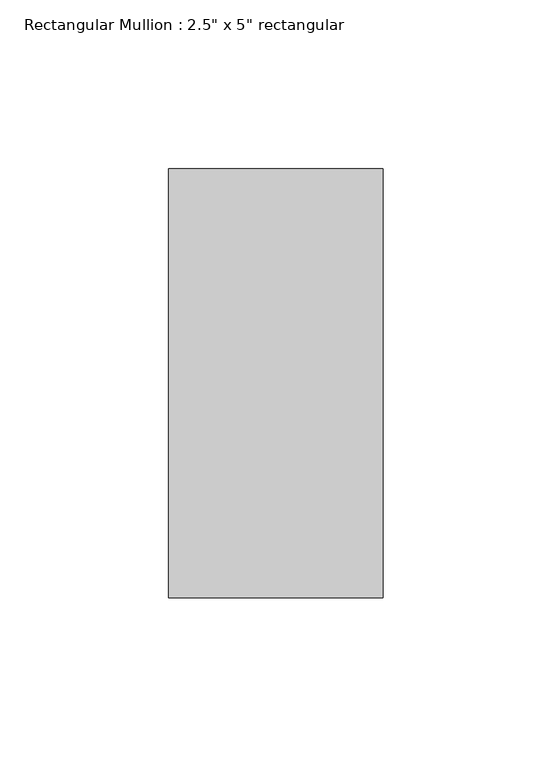
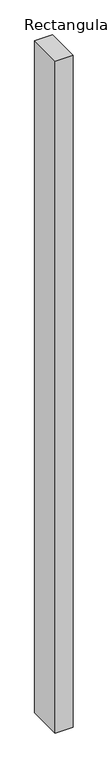
"""IFC4 building model written with IfcOpenShell, lengths in millimetres: member geometry."""

from ifc_helpers import new_model, si_unit, frame, origin, place, context, project, spatial, polyline, outline, extrude, source, transform, mapped, element, save


def member_42d69148(model_context):
    return source(origin(), model_context, "Body", "SweptSolid", [
        extrude(outline(polyline([(0.0, 63.5), (0.0, -63.5), (-63.5, -63.5), (-63.5, 63.5), (0.0, 63.5)])), frame((0.0, 0.0, -2538.6388159), z_axis=(0.0, 0.0, 1.0), x_axis=(1.0, 0.0, 0.0)), (0.0, 0.0, 1.0), 2538.6388159),
    ])


if __name__ == "__main__":
    model = new_model("IFC4")
    model_context = context("Model", 3, world=origin())
    ifc_project = project(units=[si_unit("LENGTHUNIT", "METRE", prefix="MILLI")], contexts=[model_context])
    site = spatial("IfcSite", under=ifc_project)
    building = spatial("IfcBuilding", under=site)
    placement = place(None, origin())
    member_shape = member_42d69148(model_context)
    element("IfcMember", 1, ObjectType="Rectangular Mullion : 2.5\" x 5\" rectangular", at=placement, inside=building, context=model_context, shape_type="MappedRepresentation", body=[
        mapped(member_shape, transform((0.0, 0.0, 0.0), x_axis=(1.0, 0.0, 0.0), y_axis=(0.0, 1.0, 0.0), z_axis=(0.0, 0.0, 1.0))),
    ])
    save(model, "model.ifc")

# Revit data of these elements
# Type "Rectangular Mullion : 2.5\" x 5\" rectangular"
#   built-in parameter 1007304 = 0.416667 (stored number, unit not read)
#   built-in parameter 1007301 = 0.104167 (stored number, unit not read)
#   built-in parameter 1007300 = 0.104167 (stored number, unit not read)
# Element 1 (IfcMember, "Rectangular Mullion : 2.5\" x 5\" rectangular")
#   Materials on its faces: "Aluminum"
# Materials
#   "Aluminum": class "Metal", colour RGB 247 247 247, transparency 0, Description = "Aluminum 6061", Cost = 0
